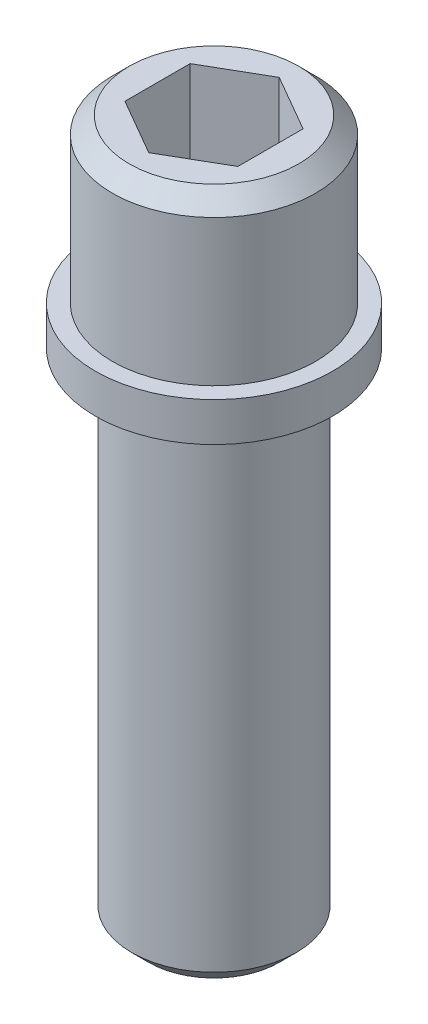
SolidWorks part; units mm, degrees
material "Plain Carbon Steel"
ref_plane "Front Plane" through (0, 0, 0) normal (0, 0, 1) x (1, 0, 0)
ref_plane "Top Plane" through (0, 0, 0) normal (0, 1, 0) x (1, 0, 0)
ref_plane "Right Plane" through (0, 0, 0) normal (1, 0, 0) x (0, 0, -1)
sketch "Shank Sketch Ø9.7" plane through (0, 0, 0) normal (0, 1, 0) x (1, 0, 0)
  circle A0 centre (0, 0) radius 4.85
  dimension "D1" = 9.7
extrude "Shank Ø9.7x29.5" add sketch "Shank Sketch Ø9.7" along normal blind 29.5
sketch "Flange Sketch Ø17.3" plane through (0, 29.5, 0) normal (0, 1, 0) x (1, 0, 0)
  circle A0 centre (0, 0) radius 7
  dimension "D1" = 14
extrude "Flange Ø17.3x2.3" add sketch "Flange Sketch Ø17.3" along normal blind 2.3
sketch "Head Sketch Ø12" plane through (0, 31.8, 0) normal (0, 1, 0) x (1, 0, 0)
  circle A0 centre (0, 0) radius 6
  dimension "D1" = 12
extrude "Head Ø12x9.6" add sketch "Head Sketch Ø12" along normal blind 9.6
sketch "Hex Socket Sketch 7.7" plane through (0, 41.4, 0) normal (0, 1, 0) x (1, 0, 0)
  line L1 (0, 3.85) -> (-3.3342, 1.925)
  line L2 (-3.3342, 1.925) -> (-3.3342, -1.925)
  line L3 (-3.3342, -1.925) -> (0, -3.85)
  line L4 (0, -3.85) -> (3.3342, -1.925)
  line L5 (3.3342, -1.925) -> (3.3342, 1.925)
  line L6 (3.3342, 1.925) -> (0, 3.85)
  circle A0 centre (0, 0) radius 3.85 construction
  dimension "D1" = 7.7
extrude "Hex Socket 7.7x9.6 Deep" cut sketch "Hex Socket Sketch 7.7" against normal blind 9.6
chamfer "Head Top Chamfer 1x45" distance 1 angle 45 1 edges at (0, 41.4, 6)
chamfer "Shank End Chamfer 1x45" distance 1 angle 45 1 edges at (0, 0, 4.85)
